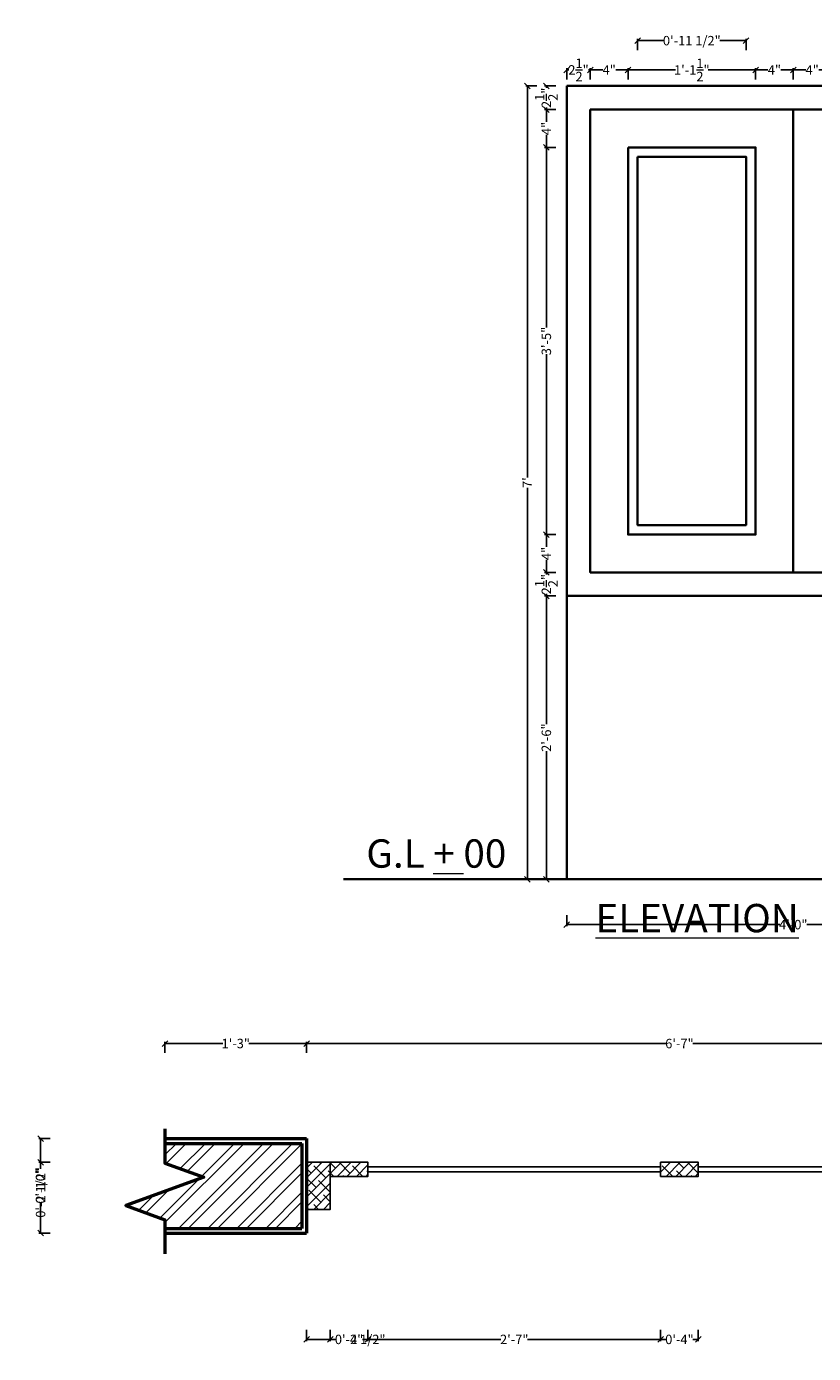
# Model space of a CAD drawing. Units: inches. Extents: x -54 to 163, y -154 to 48.
# Tile 1 of 3: x -54 to 30, y -112 to 28. Entities that reach past the tile are written whole.
import ezdxf

# ---------------------------------------------------------------- set-up
doc = ezdxf.new("R2010")
doc.units = ezdxf.units.IN
doc.header["$MEASUREMENT"] = 0
for name, color, linetype, lineweight in [('A-ANNO-DIMS', 2, 'Continuous', 18), ('A-ANNO-TEXT', 3, 'Continuous', 18), ('A-ELEV', 7, 'Continuous', 35), ('A-GLAZ', 4, 'Continuous', 25), ('A-GLAZ-PATT', 9, 'Continuous', 13), ('A-WALL', 7, 'Continuous', 50), ('A-WALL-PATT', 8, 'Continuous', 18)]:
    doc.layers.add(name, color=color, linetype=linetype, lineweight=lineweight)
doc.styles.get("Standard").update_dxf_attribs({"font": 'arial.ttf'})
doc.dimstyles.get("Standard").update_dxf_attribs({"dimtxt": 1, "dimasz": 0.6, "dimexe": 0.18, "dimexo": 0.0625, "dimgap": 0.09, "dimtad": 0, "dimdec": 1, "dimzin": 0, "dimdsep": 46, "dimlunit": 4, "dimtxsty": 'Standard', "dimblk": 'OBLIQUE', "dimcen": 0.09, "dimadec": 0, "dimazin": 0, "dimtfac": 1, "dimtdec": 1, "dimtofl": 0, "dimtmove": 0, "dimatfit": 3, "dimfxl": 1, "dimfxlon": 1, "dimtolj": 1, "dimtzin": 0, "dimarcsym": 0})

# ---------------------------------------------------------------- blocks, each defined once
blk = doc.blocks.new('_Oblique')
at = {"color": 0, "linetype": 'ByBlock', "lineweight": -2}
blk.add_line((-0.5, -0.5), (0.5, 0.5), dxfattribs=at)
blk = doc.blocks.new('*D2')
at = {"layer": 'A-ANNO-DIMS', "color": 0, "lineweight": -2, "transparency": 16777216}
for p, q in [((3.48, 22.51), (3.48, 23.69)), ((3.48, 23.51), (3.69, 23.51)), ((5.98, 23.51), (5.77, 23.51)), ((5.98, 22.51), (5.98, 23.69))]:
    blk.add_line(p, q, dxfattribs=at)
at = {"layer": 'Defpoints', "color": 0, "transparency": 16777216}
for p in [(5.98, 23.51), (3.48, 21.81), (5.98, 19.31)]:
    blk.add_point(p, dxfattribs=at)
at = {"layer": 'A-ANNO-DIMS', "color": 0, "lineweight": -2, "transparency": 16777216, "xscale": 0.6, "yscale": 0.6, "zscale": 0.6, "rotation": 180}
blk.add_blockref('_Oblique', (3.48, 23.51), dxfattribs=at)
at = {"layer": 'A-ANNO-DIMS', "color": 0, "lineweight": -2, "transparency": 16777216, "xscale": 0.6, "yscale": 0.6, "zscale": 0.6}
blk.add_blockref('_Oblique', (5.98, 23.51), dxfattribs=at)
at = {"layer": 'A-ANNO-DIMS', "color": 0, "transparency": 16777216, "insert": (4.73, 23.51), "char_height": 1, "attachment_point": 5}
blk.add_mtext('\\A1;2{\\H1x;\\S1/2;}"', dxfattribs=at)
blk = doc.blocks.new('*D3')
at = {"layer": 'A-ANNO-DIMS', "color": 0, "lineweight": -2, "transparency": 16777216}
for p, q in [((5.98, 22.51), (5.98, 23.69)), ((5.98, 23.51), (7.3, 23.51)), ((9.98, 23.51), (8.67, 23.51)), ((9.98, 22.51), (9.98, 23.69))]:
    blk.add_line(p, q, dxfattribs=at)
at = {"layer": 'Defpoints', "color": 0, "transparency": 16777216}
for p in [(9.98, 23.51), (5.98, 19.31), (9.98, 15.31)]:
    blk.add_point(p, dxfattribs=at)
at = {"layer": 'A-ANNO-DIMS', "color": 0, "lineweight": -2, "transparency": 16777216, "xscale": 0.6, "yscale": 0.6, "zscale": 0.6, "rotation": 180}
blk.add_blockref('_Oblique', (5.98, 23.51), dxfattribs=at)
at = {"layer": 'A-ANNO-DIMS', "color": 0, "lineweight": -2, "transparency": 16777216, "xscale": 0.6, "yscale": 0.6, "zscale": 0.6}
blk.add_blockref('_Oblique', (9.98, 23.51), dxfattribs=at)
at = {"layer": 'A-ANNO-DIMS', "color": 0, "transparency": 16777216, "insert": (7.98, 23.51), "char_height": 1, "attachment_point": 5}
blk.add_mtext('\\A1;4"', dxfattribs=at)
blk = doc.blocks.new('*D4')
at = {"layer": 'A-ANNO-DIMS', "color": 0, "lineweight": -2, "transparency": 16777216}
for p, q in [((9.98, 22.51), (9.98, 23.69)), ((9.98, 23.51), (14.99, 23.51)), ((23.48, 23.51), (18.47, 23.51)), ((23.48, 22.51), (23.48, 23.69))]:
    blk.add_line(p, q, dxfattribs=at)
at = {"layer": 'Defpoints', "color": 0, "transparency": 16777216}
for p in [(23.48, 23.51), (9.98, 15.31), (23.48, 15.31)]:
    blk.add_point(p, dxfattribs=at)
at = {"layer": 'A-ANNO-DIMS', "color": 0, "lineweight": -2, "transparency": 16777216, "xscale": 0.6, "yscale": 0.6, "zscale": 0.6, "rotation": 180}
blk.add_blockref('_Oblique', (9.98, 23.51), dxfattribs=at)
at = {"layer": 'A-ANNO-DIMS', "color": 0, "lineweight": -2, "transparency": 16777216, "xscale": 0.6, "yscale": 0.6, "zscale": 0.6}
blk.add_blockref('_Oblique', (23.48, 23.51), dxfattribs=at)
at = {"layer": 'A-ANNO-DIMS', "color": 0, "transparency": 16777216, "insert": (16.73, 23.51), "char_height": 1, "attachment_point": 5}
blk.add_mtext('\\A1;1\'-1{\\H1x;\\S1/2;}"', dxfattribs=at)
blk = doc.blocks.new('*D5')
at = {"layer": 'A-ANNO-DIMS', "color": 0, "lineweight": -2, "transparency": 16777216}
for p, q in [((23.48, 22.51), (23.48, 23.69)), ((23.48, 23.51), (24.8, 23.51)), ((27.48, 23.51), (26.17, 23.51)), ((27.48, 22.51), (27.48, 23.69))]:
    blk.add_line(p, q, dxfattribs=at)
at = {"layer": 'Defpoints', "color": 0, "transparency": 16777216}
for p in [(27.48, 23.51), (23.48, 15.31), (27.48, 15.31)]:
    blk.add_point(p, dxfattribs=at)
at = {"layer": 'A-ANNO-DIMS', "color": 0, "lineweight": -2, "transparency": 16777216, "xscale": 0.6, "yscale": 0.6, "zscale": 0.6, "rotation": 180}
blk.add_blockref('_Oblique', (23.48, 23.51), dxfattribs=at)
at = {"layer": 'A-ANNO-DIMS', "color": 0, "lineweight": -2, "transparency": 16777216, "xscale": 0.6, "yscale": 0.6, "zscale": 0.6}
blk.add_blockref('_Oblique', (27.48, 23.51), dxfattribs=at)
at = {"layer": 'A-ANNO-DIMS', "color": 0, "transparency": 16777216, "insert": (25.48, 23.51), "char_height": 1, "attachment_point": 5}
blk.add_mtext('\\A1;4"', dxfattribs=at)
blk = doc.blocks.new('*D6')
at = {"layer": 'A-ANNO-DIMS', "color": 0, "lineweight": -2, "transparency": 16777216}
for p, q in [((27.48, 22.51), (27.48, 23.69)), ((27.48, 23.51), (28.8, 23.51)), ((31.48, 23.51), (30.17, 23.51)), ((31.48, 22.51), (31.48, 23.69))]:
    blk.add_line(p, q, dxfattribs=at)
at = {"layer": 'Defpoints', "color": 0, "transparency": 16777216}
for p in [(31.48, 23.51), (27.48, 15.31), (31.48, 15.31)]:
    blk.add_point(p, dxfattribs=at)
at = {"layer": 'A-ANNO-DIMS', "color": 0, "lineweight": -2, "transparency": 16777216, "xscale": 0.6, "yscale": 0.6, "zscale": 0.6, "rotation": 180}
blk.add_blockref('_Oblique', (27.48, 23.51), dxfattribs=at)
at = {"layer": 'A-ANNO-DIMS', "color": 0, "lineweight": -2, "transparency": 16777216, "xscale": 0.6, "yscale": 0.6, "zscale": 0.6}
blk.add_blockref('_Oblique', (31.48, 23.51), dxfattribs=at)
at = {"layer": 'A-ANNO-DIMS', "color": 0, "transparency": 16777216, "insert": (29.48, 23.51), "char_height": 1, "attachment_point": 5}
blk.add_mtext('\\A1;4"', dxfattribs=at)
blk = doc.blocks.new('*D10')
at = {"layer": 'A-ANNO-DIMS', "color": 0, "lineweight": -2, "transparency": 16777216}
for p, q in [((2.32, 21.81), (1.14, 21.81)), ((1.32, 21.81), (1.32, 21.6)), ((2.32, 19.31), (1.14, 19.31)), ((1.32, 19.31), (1.32, 19.53))]:
    blk.add_line(p, q, dxfattribs=at)
at = {"layer": 'Defpoints', "color": 0, "transparency": 16777216}
for p in [(1.32, 21.81), (5.98, 21.81), (5.98, 19.31)]:
    blk.add_point(p, dxfattribs=at)
at = {"layer": 'A-ANNO-DIMS', "color": 0, "lineweight": -2, "transparency": 16777216, "xscale": 0.6, "yscale": 0.6, "zscale": 0.6}
for p, rotation in [((1.32, 21.81), 90), ((1.32, 19.31), 270)]:
    blk.add_blockref('_Oblique', p, dxfattribs=dict(at, rotation=rotation))
at = {"layer": 'A-ANNO-DIMS', "color": 0, "transparency": 16777216, "insert": (1.32, 20.56), "char_height": 1, "attachment_point": 5, "rotation": 90}
blk.add_mtext('\\A1;2{\\H1x;\\S1/2;}"', dxfattribs=at)
blk = doc.blocks.new('*D11')
at = {"layer": 'A-ANNO-DIMS', "color": 0, "lineweight": -2, "transparency": 16777216}
for p, q in [((2.32, 19.31), (1.14, 19.31)), ((1.32, 19.31), (1.32, 18)), ((1.32, 15.31), (1.32, 16.63)), ((2.32, 15.31), (1.14, 15.31))]:
    blk.add_line(p, q, dxfattribs=at)
at = {"layer": 'Defpoints', "color": 0, "transparency": 16777216}
for p in [(1.32, 19.31), (9.98, 19.31), (9.98, 15.31)]:
    blk.add_point(p, dxfattribs=at)
at = {"layer": 'A-ANNO-DIMS', "color": 0, "lineweight": -2, "transparency": 16777216, "xscale": 0.6, "yscale": 0.6, "zscale": 0.6}
for p, rotation in [((1.32, 19.31), 90), ((1.32, 15.31), 270)]:
    blk.add_blockref('_Oblique', p, dxfattribs=dict(at, rotation=rotation))
at = {"layer": 'A-ANNO-DIMS', "color": 0, "transparency": 16777216, "insert": (1.32, 17.31), "char_height": 1, "attachment_point": 5, "rotation": 90}
blk.add_mtext('\\A1;4"', dxfattribs=at)
blk = doc.blocks.new('*D12')
at = {"layer": 'A-ANNO-DIMS', "color": 0, "lineweight": -2, "transparency": 16777216}
for p, q in [((2.32, 15.31), (1.14, 15.31)), ((1.32, 15.31), (1.32, -3.77)), ((1.32, -25.69), (1.32, -6.6)), ((2.32, -25.69), (1.14, -25.69))]:
    blk.add_line(p, q, dxfattribs=at)
at = {"layer": 'Defpoints', "color": 0, "transparency": 16777216}
for p in [(9.98, 15.31), (1.32, -25.69), (9.98, -25.69)]:
    blk.add_point(p, dxfattribs=at)
at = {"layer": 'A-ANNO-DIMS', "color": 0, "lineweight": -2, "transparency": 16777216, "xscale": 0.6, "yscale": 0.6, "zscale": 0.6}
for p, rotation in [((1.32, 15.31), 90), ((1.32, -25.69), 270)]:
    blk.add_blockref('_Oblique', p, dxfattribs=dict(at, rotation=rotation))
at = {"layer": 'A-ANNO-DIMS', "color": 0, "transparency": 16777216, "insert": (1.32, -5.19), "char_height": 1, "attachment_point": 5, "rotation": 90}
blk.add_mtext('\\A1;3\'-5"', dxfattribs=at)
blk = doc.blocks.new('*D13')
at = {"layer": 'A-ANNO-DIMS', "color": 0, "lineweight": -2, "transparency": 16777216}
for p, q in [((2.32, -25.69), (1.14, -25.69)), ((1.32, -25.69), (1.32, -27)), ((1.32, -29.69), (1.32, -28.37)), ((2.32, -29.69), (1.14, -29.69))]:
    blk.add_line(p, q, dxfattribs=at)
at = {"layer": 'Defpoints', "color": 0, "transparency": 16777216}
for p in [(10.03, -25.69), (1.32, -29.69), (10.03, -29.69)]:
    blk.add_point(p, dxfattribs=at)
at = {"layer": 'A-ANNO-DIMS', "color": 0, "lineweight": -2, "transparency": 16777216, "xscale": 0.6, "yscale": 0.6, "zscale": 0.6}
for p, rotation in [((1.32, -25.69), 90), ((1.32, -29.69), 270)]:
    blk.add_blockref('_Oblique', p, dxfattribs=dict(at, rotation=rotation))
at = {"layer": 'A-ANNO-DIMS', "color": 0, "transparency": 16777216, "insert": (1.32, -27.69), "char_height": 1, "attachment_point": 5, "rotation": 90}
blk.add_mtext('\\A1;4"', dxfattribs=at)
blk = doc.blocks.new('*D14')
at = {"layer": 'A-ANNO-DIMS', "color": 0, "lineweight": -2, "transparency": 16777216}
for p, q in [((2.32, -29.69), (1.14, -29.69)), ((1.32, -29.69), (1.32, -29.9)), ((2.32, -32.19), (1.14, -32.19)), ((1.32, -32.19), (1.32, -31.97))]:
    blk.add_line(p, q, dxfattribs=at)
at = {"layer": 'Defpoints', "color": 0, "transparency": 16777216}
for p in [(1.32, -29.69), (5.98, -29.69), (6.04, -32.19)]:
    blk.add_point(p, dxfattribs=at)
at = {"layer": 'A-ANNO-DIMS', "color": 0, "lineweight": -2, "transparency": 16777216, "xscale": 0.6, "yscale": 0.6, "zscale": 0.6}
for p, rotation in [((1.32, -29.69), 90), ((1.32, -32.19), 270)]:
    blk.add_blockref('_Oblique', p, dxfattribs=dict(at, rotation=rotation))
at = {"layer": 'A-ANNO-DIMS', "color": 0, "transparency": 16777216, "insert": (1.32, -30.94), "char_height": 1, "attachment_point": 5, "rotation": 90}
blk.add_mtext('\\A1;2{\\H1x;\\S1/2;}"', dxfattribs=at)
blk = doc.blocks.new('*D15')
at = {"layer": 'A-ANNO-DIMS', "color": 0, "lineweight": -2, "transparency": 16777216}
for p, q in [((2.32, -32.19), (1.14, -32.19)), ((1.32, -32.19), (1.32, -45.76)), ((1.32, -62.19), (1.32, -48.61)), ((2.32, -62.19), (1.14, -62.19))]:
    blk.add_line(p, q, dxfattribs=at)
at = {"layer": 'Defpoints', "color": 0, "transparency": 16777216}
for p in [(3.48, -32.19), (1.32, -62.19), (3.48, -62.19)]:
    blk.add_point(p, dxfattribs=at)
at = {"layer": 'A-ANNO-DIMS', "color": 0, "lineweight": -2, "transparency": 16777216, "xscale": 0.6, "yscale": 0.6, "zscale": 0.6}
for p, rotation in [((1.32, -32.19), 90), ((1.32, -62.19), 270)]:
    blk.add_blockref('_Oblique', p, dxfattribs=dict(at, rotation=rotation))
at = {"layer": 'A-ANNO-DIMS', "color": 0, "transparency": 16777216, "insert": (1.32, -47.19), "char_height": 1, "attachment_point": 5, "rotation": 90}
blk.add_mtext('\\A1;2\'-6"', dxfattribs=at)
blk = doc.blocks.new('*D16')
at = {"layer": 'A-ANNO-DIMS', "color": 0, "lineweight": -2, "transparency": 16777216}
for p, q in [((0.31, 21.81), (-0.87, 21.81)), ((-0.69, 21.81), (-0.69, -19.64)), ((-0.69, -62.19), (-0.69, -20.73)), ((0.31, -62.19), (-0.87, -62.19))]:
    blk.add_line(p, q, dxfattribs=at)
at = {"layer": 'Defpoints', "color": 0, "transparency": 16777216}
for p in [(-0.69, 21.81), (3.48, 21.81), (3.48, -62.19)]:
    blk.add_point(p, dxfattribs=at)
at = {"layer": 'A-ANNO-DIMS', "color": 0, "lineweight": -2, "transparency": 16777216, "xscale": 0.6, "yscale": 0.6, "zscale": 0.6}
for p, rotation in [((-0.69, 21.81), 90), ((-0.69, -62.19), 270)]:
    blk.add_blockref('_Oblique', p, dxfattribs=dict(at, rotation=rotation))
at = {"layer": 'A-ANNO-DIMS', "color": 0, "transparency": 16777216, "insert": (-0.69, -20.19), "char_height": 1, "attachment_point": 5, "rotation": 90}
blk.add_mtext("\\A1;7'", dxfattribs=at)
blk = doc.blocks.new('*D18')
at = {"layer": 'A-ANNO-DIMS', "color": 0, "lineweight": -2, "transparency": 16777216}
for p, q in [((3.48, -65.99), (3.48, -67.17)), ((51.48, -65.99), (51.48, -67.17)), ((3.48, -66.99), (26.04, -66.99)), ((51.48, -66.99), (28.92, -66.99))]:
    blk.add_line(p, q, dxfattribs=at)
at = {"layer": 'Defpoints', "color": 0, "transparency": 16777216}
for p in [(3.48, -62.19), (51.48, -62.19), (51.48, -66.99)]:
    blk.add_point(p, dxfattribs=at)
at = {"layer": 'A-ANNO-DIMS', "color": 0, "lineweight": -2, "transparency": 16777216, "xscale": 0.6, "yscale": 0.6, "zscale": 0.6, "rotation": 180}
blk.add_blockref('_Oblique', (3.48, -66.99), dxfattribs=at)
at = {"layer": 'A-ANNO-DIMS', "color": 0, "lineweight": -2, "transparency": 16777216, "xscale": 0.6, "yscale": 0.6, "zscale": 0.6}
blk.add_blockref('_Oblique', (51.48, -66.99), dxfattribs=at)
at = {"layer": 'A-ANNO-DIMS', "color": 0, "transparency": 16777216, "insert": (27.48, -66.99), "char_height": 1, "attachment_point": 5}
blk.add_mtext('\\A1;4\'-0"', dxfattribs=at)
blk = doc.blocks.new('*D19')
at = {"layer": 'A-ANNO-DIMS', "color": 0, "lineweight": -2, "transparency": 16777216}
for p, q in [((10.98, 25.61), (10.98, 26.79)), ((22.48, 25.61), (22.48, 26.79)), ((10.98, 26.61), (13.76, 26.61)), ((22.48, 26.61), (19.7, 26.61))]:
    blk.add_line(p, q, dxfattribs=at)
at = {"layer": 'Defpoints', "color": 0, "transparency": 16777216}
for p in [(22.48, 26.61), (10.98, 14.31), (22.48, 14.31)]:
    blk.add_point(p, dxfattribs=at)
at = {"layer": 'A-ANNO-DIMS', "color": 0, "lineweight": -2, "transparency": 16777216, "xscale": 0.6, "yscale": 0.6, "zscale": 0.6, "rotation": 180}
blk.add_blockref('_Oblique', (10.98, 26.61), dxfattribs=at)
at = {"layer": 'A-ANNO-DIMS', "color": 0, "lineweight": -2, "transparency": 16777216, "xscale": 0.6, "yscale": 0.6, "zscale": 0.6}
blk.add_blockref('_Oblique', (22.48, 26.61), dxfattribs=at)
at = {"layer": 'A-ANNO-DIMS', "color": 0, "transparency": 16777216, "insert": (16.73, 26.61), "char_height": 1, "attachment_point": 5}
blk.add_mtext('\\A1;0\'-11 1/2"', dxfattribs=at)
blk = doc.blocks.new('*D20')
at = {"layer": 'A-ANNO-DIMS', "color": 0, "lineweight": -2, "transparency": 16777216}
for p, q in [((55.28, 14.31), (56.46, 14.31)), ((56.28, 14.31), (56.28, -3.77)), ((56.28, -24.69), (56.28, -6.6)), ((55.28, -24.69), (56.46, -24.69))]:
    blk.add_line(p, q, dxfattribs=at)
at = {"layer": 'Defpoints', "color": 0, "transparency": 16777216}
for p in [(10.98, 14.31), (10.98, -24.69), (56.28, -24.69)]:
    blk.add_point(p, dxfattribs=at)
at = {"layer": 'A-ANNO-DIMS', "color": 0, "lineweight": -2, "transparency": 16777216, "xscale": 0.6, "yscale": 0.6, "zscale": 0.6}
for p, rotation in [((56.28, 14.31), 90), ((56.28, -24.69), 270)]:
    blk.add_blockref('_Oblique', p, dxfattribs=dict(at, rotation=rotation))
at = {"layer": 'A-ANNO-DIMS', "color": 0, "transparency": 16777216, "insert": (56.28, -5.19), "char_height": 1, "attachment_point": 5, "rotation": 90}
blk.add_mtext('\\A1;3\'-3"', dxfattribs=at)
blk = doc.blocks.new('*D33')
at = {"layer": 'A-ANNO-DIMS', "color": 0, "lineweight": -2, "transparency": 16777216}
for p, q in [((-39.08, -80.58), (-39.08, -79.4)), ((-39.08, -79.58), (-32.96, -79.58)), ((-24.08, -79.58), (-30.21, -79.58)), ((-24.08, -80.58), (-24.08, -79.4))]:
    blk.add_line(p, q, dxfattribs=at)
at = {"layer": 'Defpoints', "color": 0, "transparency": 16777216}
for p in [(-24.08, -79.58), (-39.08, -89.65), (-24.08, -89.65)]:
    blk.add_point(p, dxfattribs=at)
at = {"layer": 'A-ANNO-DIMS', "color": 0, "lineweight": -2, "transparency": 16777216, "xscale": 0.6, "yscale": 0.6, "zscale": 0.6, "rotation": 180}
blk.add_blockref('_Oblique', (-39.08, -79.58), dxfattribs=at)
at = {"layer": 'A-ANNO-DIMS', "color": 0, "lineweight": -2, "transparency": 16777216, "xscale": 0.6, "yscale": 0.6, "zscale": 0.6}
blk.add_blockref('_Oblique', (-24.08, -79.58), dxfattribs=at)
at = {"layer": 'A-ANNO-DIMS', "color": 0, "transparency": 16777216, "insert": (-31.58, -79.58), "char_height": 1, "attachment_point": 5}
blk.add_mtext('\\A1;1\'-3"', dxfattribs=at)
blk = doc.blocks.new('*D34')
at = {"layer": 'A-ANNO-DIMS', "color": 0, "lineweight": -2, "transparency": 16777216}
for p, q in [((-24.08, -80.58), (-24.08, -79.4)), ((-24.08, -79.58), (13.99, -79.58)), ((54.92, -79.58), (16.84, -79.58)), ((54.92, -80.58), (54.92, -79.4))]:
    blk.add_line(p, q, dxfattribs=at)
at = {"layer": 'Defpoints', "color": 0, "transparency": 16777216}
for p in [(54.92, -79.58), (-24.08, -89.65), (54.92, -89.65)]:
    blk.add_point(p, dxfattribs=at)
at = {"layer": 'A-ANNO-DIMS', "color": 0, "lineweight": -2, "transparency": 16777216, "xscale": 0.6, "yscale": 0.6, "zscale": 0.6, "rotation": 180}
blk.add_blockref('_Oblique', (-24.08, -79.58), dxfattribs=at)
at = {"layer": 'A-ANNO-DIMS', "color": 0, "lineweight": -2, "transparency": 16777216, "xscale": 0.6, "yscale": 0.6, "zscale": 0.6}
blk.add_blockref('_Oblique', (54.92, -79.58), dxfattribs=at)
at = {"layer": 'A-ANNO-DIMS', "color": 0, "transparency": 16777216, "insert": (15.42, -79.58), "char_height": 1, "attachment_point": 5}
blk.add_mtext('\\A1;6\'-7"', dxfattribs=at)
blk = doc.blocks.new('*D36')
at = {"layer": 'A-ANNO-DIMS', "color": 0, "lineweight": -2, "transparency": 16777216}
for p, q in [((-24.08, -109.91), (-24.08, -111.09)), ((-24.08, -110.91), (-21.58, -110.91)), ((-21.58, -109.91), (-21.58, -111.09)), ((-21.58, -110.91), (-20.98, -110.91))]:
    blk.add_line(p, q, dxfattribs=at)
at = {"layer": 'Defpoints', "color": 0, "transparency": 16777216}
for p in [(-24.08, -97.15), (-21.58, -97.15), (-21.58, -110.91)]:
    blk.add_point(p, dxfattribs=at)
at = {"layer": 'A-ANNO-DIMS', "color": 0, "lineweight": -2, "transparency": 16777216, "xscale": 0.6, "yscale": 0.6, "zscale": 0.6, "rotation": 180}
blk.add_blockref('_Oblique', (-24.08, -110.91), dxfattribs=at)
at = {"layer": 'A-ANNO-DIMS', "color": 0, "lineweight": -2, "transparency": 16777216, "xscale": 0.6, "yscale": 0.6, "zscale": 0.6}
blk.add_blockref('_Oblique', (-21.58, -110.91), dxfattribs=at)
at = {"layer": 'A-ANNO-DIMS', "color": 0, "transparency": 16777216, "insert": (-18.4, -110.91), "char_height": 1, "attachment_point": 5}
blk.add_mtext('\\A1;0\'-2 1/2"', dxfattribs=at)
blk = doc.blocks.new('*D37')
at = {"layer": 'A-ANNO-DIMS', "color": 0, "lineweight": -2, "transparency": 16777216}
for p, q in [((-21.58, -109.91), (-21.58, -111.09)), ((-21.58, -110.91), (-21, -110.91)), ((-17.58, -110.91), (-18.17, -110.91)), ((-17.58, -109.91), (-17.58, -111.09))]:
    blk.add_line(p, q, dxfattribs=at)
at = {"layer": 'Defpoints', "color": 0, "transparency": 16777216}
for p in [(-21.58, -93.65), (-17.58, -93.65), (-17.58, -110.91)]:
    blk.add_point(p, dxfattribs=at)
at = {"layer": 'A-ANNO-DIMS', "color": 0, "lineweight": -2, "transparency": 16777216, "xscale": 0.6, "yscale": 0.6, "zscale": 0.6, "rotation": 180}
blk.add_blockref('_Oblique', (-21.58, -110.91), dxfattribs=at)
at = {"layer": 'A-ANNO-DIMS', "color": 0, "lineweight": -2, "transparency": 16777216, "xscale": 0.6, "yscale": 0.6, "zscale": 0.6}
blk.add_blockref('_Oblique', (-17.58, -110.91), dxfattribs=at)
at = {"layer": 'A-ANNO-DIMS', "color": 0, "transparency": 16777216, "insert": (-19.58, -110.91), "char_height": 1, "attachment_point": 5}
blk.add_mtext('\\A1;0\'-4"', dxfattribs=at)
blk = doc.blocks.new('*D38')
at = {"layer": 'A-ANNO-DIMS', "color": 0, "lineweight": -2, "transparency": 16777216}
for p, q in [((-17.58, -109.91), (-17.58, -111.09)), ((-17.58, -110.91), (-3.51, -110.91)), ((13.42, -110.91), (-0.66, -110.91)), ((13.42, -109.91), (13.42, -111.09))]:
    blk.add_line(p, q, dxfattribs=at)
at = {"layer": 'Defpoints', "color": 0, "transparency": 16777216}
for p in [(-17.58, -93.65), (13.42, -93.65), (13.42, -110.91)]:
    blk.add_point(p, dxfattribs=at)
at = {"layer": 'A-ANNO-DIMS', "color": 0, "lineweight": -2, "transparency": 16777216, "xscale": 0.6, "yscale": 0.6, "zscale": 0.6, "rotation": 180}
blk.add_blockref('_Oblique', (-17.58, -110.91), dxfattribs=at)
at = {"layer": 'A-ANNO-DIMS', "color": 0, "lineweight": -2, "transparency": 16777216, "xscale": 0.6, "yscale": 0.6, "zscale": 0.6}
blk.add_blockref('_Oblique', (13.42, -110.91), dxfattribs=at)
at = {"layer": 'A-ANNO-DIMS', "color": 0, "transparency": 16777216, "insert": (-2.08, -110.91), "char_height": 1, "attachment_point": 5}
blk.add_mtext('\\A1;2\'-7"', dxfattribs=at)
blk = doc.blocks.new('*D39')
at = {"layer": 'A-ANNO-DIMS', "color": 0, "lineweight": -2, "transparency": 16777216}
for p, q in [((13.42, -109.91), (13.42, -111.09)), ((13.42, -110.91), (14, -110.91)), ((17.42, -110.91), (16.83, -110.91)), ((17.42, -109.91), (17.42, -111.09))]:
    blk.add_line(p, q, dxfattribs=at)
at = {"layer": 'Defpoints', "color": 0, "transparency": 16777216}
for p in [(13.42, -93.65), (17.42, -93.65), (17.42, -110.91)]:
    blk.add_point(p, dxfattribs=at)
at = {"layer": 'A-ANNO-DIMS', "color": 0, "lineweight": -2, "transparency": 16777216, "xscale": 0.6, "yscale": 0.6, "zscale": 0.6, "rotation": 180}
blk.add_blockref('_Oblique', (13.42, -110.91), dxfattribs=at)
at = {"layer": 'A-ANNO-DIMS', "color": 0, "lineweight": -2, "transparency": 16777216, "xscale": 0.6, "yscale": 0.6, "zscale": 0.6}
blk.add_blockref('_Oblique', (17.42, -110.91), dxfattribs=at)
at = {"layer": 'A-ANNO-DIMS', "color": 0, "transparency": 16777216, "insert": (15.42, -110.91), "char_height": 1, "attachment_point": 5}
blk.add_mtext('\\A1;0\'-4"', dxfattribs=at)
blk = doc.blocks.new('*D40')
at = {"layer": 'A-ANNO-DIMS', "color": 0, "lineweight": -2, "transparency": 16777216}
for p, q in [((-51.26, -89.65), (-52.44, -89.65)), ((-52.26, -89.65), (-52.26, -92.85)), ((-52.26, -99.65), (-52.26, -96.46)), ((-51.26, -99.65), (-52.44, -99.65))]:
    blk.add_line(p, q, dxfattribs=at)
at = {"layer": 'Defpoints', "color": 0, "transparency": 16777216}
for p in [(-39.08, -89.65), (-52.26, -99.65), (-39.08, -99.65)]:
    blk.add_point(p, dxfattribs=at)
at = {"layer": 'A-ANNO-DIMS', "color": 0, "lineweight": -2, "transparency": 16777216, "xscale": 0.6, "yscale": 0.6, "zscale": 0.6}
for p, rotation in [((-52.26, -89.65), 90), ((-52.26, -99.65), 270)]:
    blk.add_blockref('_Oblique', p, dxfattribs=dict(at, rotation=rotation))
at = {"layer": 'A-ANNO-DIMS', "color": 0, "transparency": 16777216, "insert": (-52.26, -94.65), "char_height": 1, "attachment_point": 5, "rotation": 90}
blk.add_mtext('\\A1;0\'-10"', dxfattribs=at)
blk = doc.blocks.new('*D41')
at = {"layer": 'A-ANNO-DIMS', "color": 0, "lineweight": -2, "transparency": 16777216}
for p, q in [((-51.26, -89.65), (-52.44, -89.65)), ((-52.26, -89.65), (-52.26, -92.15)), ((-51.26, -92.15), (-52.44, -92.15)), ((-52.26, -92.15), (-52.26, -92.75))]:
    blk.add_line(p, q, dxfattribs=at)
at = {"layer": 'Defpoints', "color": 0, "transparency": 16777216}
for p in [(54.92, -89.65), (-52.26, -92.15), (52.42, -92.15)]:
    blk.add_point(p, dxfattribs=at)
at = {"layer": 'A-ANNO-DIMS', "color": 0, "lineweight": -2, "transparency": 16777216, "xscale": 0.6, "yscale": 0.6, "zscale": 0.6}
for p, rotation in [((-52.26, -89.65), 90), ((-52.26, -92.15), 270)]:
    blk.add_blockref('_Oblique', p, dxfattribs=dict(at, rotation=rotation))
at = {"layer": 'A-ANNO-DIMS', "color": 0, "transparency": 16777216, "insert": (-52.26, -95.34), "char_height": 1, "attachment_point": 5, "rotation": 90}
blk.add_mtext('\\A1;0\'-2 1/2"', dxfattribs=at)
blk = doc.blocks.new('*D42')
at = {"layer": 'A-ANNO-DIMS', "color": 0, "lineweight": -2, "transparency": 16777216}
for p, q in [((82.09, -92.15), (83.27, -92.15)), ((83.09, -92.15), (83.09, -93.24)), ((83.09, -97.15), (83.09, -96.07)), ((82.09, -97.15), (83.27, -97.15))]:
    blk.add_line(p, q, dxfattribs=at)
at = {"layer": 'Defpoints', "color": 0, "transparency": 16777216}
for p in [(-24.08, -92.15), (-24.08, -97.15), (83.09, -97.15)]:
    blk.add_point(p, dxfattribs=at)
at = {"layer": 'A-ANNO-DIMS', "color": 0, "lineweight": -2, "transparency": 16777216, "xscale": 0.6, "yscale": 0.6, "zscale": 0.6}
for p, rotation in [((83.09, -92.15), 90), ((83.09, -97.15), 270)]:
    blk.add_blockref('_Oblique', p, dxfattribs=dict(at, rotation=rotation))
at = {"layer": 'A-ANNO-DIMS', "color": 0, "transparency": 16777216, "insert": (83.09, -94.65), "char_height": 1, "attachment_point": 5, "rotation": 90}
blk.add_mtext('\\A1;0\'-5"', dxfattribs=at)

msp = doc.modelspace()

# ---------------------------------------------------------------- hatches: boundary and pattern name
at = {"layer": 'A-GLAZ-PATT'}
h = msp.add_hatch(dxfattribs=at)
h.set_pattern_fill('ANSI38', color=256, scale=5.8)
h.paths.add_polyline_path([(54.92, -92.15), (52.42, -92.15), (52.42, -97.15), (54.92, -97.15)])
h.paths.add_polyline_path([(52.42, -92.15), (48.42, -92.15), (48.42, -93.65), (52.42, -93.65)])
h.paths.add_polyline_path([(17.42, -92.15), (13.42, -92.15), (13.42, -93.65), (17.42, -93.65)])
h.paths.add_polyline_path([(-21.58, -92.15), (-24.08, -92.15), (-24.08, -97.15), (-21.58, -97.15)])
h.paths.add_polyline_path([(-17.58, -92.15), (-21.58, -92.15), (-21.58, -93.65), (-17.58, -93.65)])
at = {"layer": 'A-WALL-PATT'}
h = msp.add_hatch(dxfattribs=at)
h.set_pattern_fill('ANSI32', color=256, scale=5.8)
h.paths.add_polyline_path([(65.79, -93.74), (69.92, -92.24), (69.92, -90.15), (55.42, -90.15), (55.42, -99.15), (69.92, -99.15), (69.92, -98.24), (74.04, -96.74)])
h.paths.add_polyline_path([(-24.58, -90.15), (-39.08, -90.15), (-39.08, -92.24), (-34.96, -93.74), (-43.21, -96.74), (-39.08, -98.24), (-39.08, -99.15), (-24.58, -99.15)])

# ---------------------------------------------------------------- linework, layer by layer
at = {"layer": 'A-ELEV'}
for p, q in [((27.48, 19.31), (27.48, -29.69)), ((3.48, -32.19), (3.48, -62.19)), ((-20.18, -62.19), (51.48, -62.19))]:
    msp.add_line(p, q, dxfattribs=at)
msp.add_lwpolyline([(3.48, 21.81), (51.48, 21.81), (51.48, 19.31), (51.48, -29.69), (51.48, -32.19), (3.48, -32.19), (3.48, 21.81)], dxfattribs=at)
for points in [[(5.98, 19.31), (48.98, 19.31), (48.98, -29.69), (5.98, -29.69)], [(9.98, 15.31), (23.48, 15.31), (23.48, -25.69), (9.98, -25.69)], [(10.98, 14.31), (22.48, 14.31), (22.48, -24.69), (10.98, -24.69)]]:
    msp.add_lwpolyline(points, close=True, dxfattribs=at)
at = {"layer": 'A-GLAZ'}
for points in [[(-24.08, -92.15), (-24.08, -97.15), (-21.58, -97.15), (-21.58, -92.15)], [(-21.58, -92.15), (-21.58, -93.65), (-17.58, -93.65), (-17.58, -92.15)], [(-17.58, -92.65), (-17.58, -93.15), (13.42, -93.15), (13.42, -92.65)], [(13.42, -93.65), (13.42, -92.15), (17.42, -92.15), (17.42, -93.65)], [(48.42, -92.65), (48.42, -93.15), (17.42, -93.15), (17.42, -92.65)]]:
    msp.add_lwpolyline(points, close=True, dxfattribs=at)
at = {"layer": 'A-WALL'}
for p, q in [((-39.08, -89.65), (-24.08, -89.65)), ((-24.08, -89.65), (-24.08, -99.65)), ((-39.08, -90.15), (-24.58, -90.15)), ((-24.58, -90.15), (-24.58, -99.15)), ((-39.08, -99.15), (-24.58, -99.15)), ((-39.08, -99.65), (-24.08, -99.65))]:
    msp.add_line(p, q, dxfattribs=at)
msp.add_lwpolyline([(-39.08, -88.63), (-39.08, -92.24), (-34.96, -93.74), (-43.21, -96.74), (-39.08, -98.24), (-39.08, -101.86)], dxfattribs=at)

# ---------------------------------------------------------------- texts
at = {"layer": 'A-ANNO-TEXT', "char_height": 3, "attachment_point": 1}
for s, insert in [('G.L {\\L+} 00', (-17.75, -57.96)), ('{\\LELEVATION}', (6.53, -64.8))]:
    msp.add_mtext_dynamic_manual_height_columns(s, width=23.7975, gutter_width=1, heights=[0], dxfattribs=dict(at, insert=insert))

# ---------------------------------------------------------------- dimensions: what is measured, and where the dimension line sits
at = {"layer": 'A-ANNO-DIMS'}
for base, p1, p2, override, picture, middle in [((22.48, 26.61), (10.98, 14.31), (22.48, 14.31), {"dimdec": 1, "dimlfac": 1, "dimrnd": 0, "dimzin": 1, "dimdsep": 46, "dimlunit": 4, "dimfrac": 2}, '*D19', (16.73, 26.61)), ((5.98, 23.51), (3.48, 21.81), (5.98, 19.31), {"dimclrd": 0, "dimclre": 0, "dimclrt": 0}, '*D2', (4.73, 23.51)), ((9.98, 23.51), (5.98, 19.31), (9.98, 15.31), {"dimclrd": 0, "dimclre": 0, "dimclrt": 0}, '*D3', (7.98, 23.51)), ((23.48, 23.51), (9.98, 15.31), (23.48, 15.31), {"dimclrd": 0, "dimclre": 0, "dimclrt": 0}, '*D4', (16.73, 23.51)), ((27.48, 23.51), (23.48, 15.31), (27.48, 15.31), {"dimclrd": 0, "dimclre": 0, "dimclrt": 0}, '*D5', (25.48, 23.51)), ((31.48, 23.51), (27.48, 15.31), (31.48, 15.31), {"dimclrd": 0, "dimclre": 0, "dimclrt": 0}, '*D6', (29.48, 23.51)), ((51.48, -66.99), (3.48, -62.19), (51.48, -62.19), {"dimdec": 1, "dimlfac": 1, "dimrnd": 0, "dimzin": 1, "dimdsep": 46, "dimlunit": 4, "dimfrac": 2}, '*D18', (27.48, -66.99)), ((-24.08, -79.58), (-39.08, -89.65), (-24.08, -89.65), {"dimdec": 1, "dimlfac": 1, "dimrnd": 0, "dimzin": 1, "dimdsep": 46, "dimlunit": 4, "dimfrac": 2}, '*D33', (-31.58, -79.58)), ((54.92, -79.58), (-24.08, -89.65), (54.92, -89.65), {"dimdec": 1, "dimlfac": 1, "dimrnd": 0, "dimzin": 1, "dimdsep": 46, "dimlunit": 4, "dimfrac": 2}, '*D34', (15.42, -79.58)), ((-17.58, -110.91), (-21.58, -93.65), (-17.58, -93.65), {"dimdec": 1, "dimlfac": 1, "dimrnd": 0, "dimzin": 1, "dimdsep": 46, "dimlunit": 4, "dimfrac": 2}, '*D37', (-19.58, -110.91)), ((13.42, -110.91), (-17.58, -93.65), (13.42, -93.65), {"dimdec": 1, "dimlfac": 1, "dimrnd": 0, "dimzin": 1, "dimdsep": 46, "dimlunit": 4, "dimfrac": 2}, '*D38', (-2.08, -110.91)), ((17.42, -110.91), (13.42, -93.65), (17.42, -93.65), {"dimdec": 1, "dimlfac": 1, "dimrnd": 0, "dimzin": 1, "dimdsep": 46, "dimlunit": 4, "dimfrac": 2}, '*D39', (15.42, -110.91)), ((-21.58, -110.91), (-24.08, -97.15), (-21.58, -97.15), {"dimdec": 1, "dimlfac": 1, "dimrnd": 0, "dimzin": 1, "dimdsep": 46, "dimlunit": 4, "dimfrac": 2}, '*D36', (-18.4, -110.91))]:
    dim = msp.add_linear_dim(base=base, p1=p1, p2=p2, dimstyle='Standard', override=override, dxfattribs=at)
    dim.commit()
    dim.dimension.update_dxf_attribs({"geometry": picture, "text_midpoint": middle})
for base, p1, p2, override, picture, middle in [((-0.69, 21.81), (3.48, -62.19), (3.48, 21.81), {"dimclrd": 0, "dimclre": 0, "dimclrt": 0}, '*D16', (-0.69, -20.19)), ((1.32, 21.81), (5.98, 19.31), (5.98, 21.81), {"dimclrd": 0, "dimclre": 0, "dimclrt": 0}, '*D10', (1.32, 20.56)), ((1.32, 19.31), (9.98, 15.31), (9.98, 19.31), {"dimclrd": 0, "dimclre": 0, "dimclrt": 0}, '*D11', (1.32, 17.31)), ((1.32, -25.69), (9.98, 15.31), (9.98, -25.69), {"dimclrd": 0, "dimclre": 0, "dimclrt": 0}, '*D12', (1.32, -5.19)), ((56.28, -24.69), (10.98, 14.31), (10.98, -24.69), {"dimdec": 1, "dimlfac": 1, "dimrnd": 0, "dimzin": 1, "dimdsep": 46, "dimlunit": 4, "dimfrac": 2}, '*D20', (56.28, -5.19)), ((1.32, -29.69), (10.03, -25.69), (10.03, -29.69), {"dimclrd": 0, "dimclre": 0, "dimclrt": 0}, '*D13', (1.32, -27.69)), ((1.32, -29.69), (6.04, -32.19), (5.98, -29.69), {"dimclrd": 0, "dimclre": 0, "dimclrt": 0}, '*D14', (1.32, -30.94)), ((1.32, -62.19), (3.48, -32.19), (3.48, -62.19), {"dimclrd": 0, "dimclre": 0, "dimclrt": 0}, '*D15', (1.32, -47.19)), ((-52.26, -92.15), (54.92, -89.65), (52.42, -92.15), {"dimdec": 1, "dimlfac": 1, "dimrnd": 0, "dimzin": 1, "dimdsep": 46, "dimlunit": 4, "dimfrac": 2}, '*D41', (-52.26, -95.34)), ((-52.26, -99.65), (-39.08, -89.65), (-39.08, -99.65), {"dimdec": 1, "dimlfac": 1, "dimrnd": 0, "dimzin": 1, "dimdsep": 46, "dimlunit": 4, "dimfrac": 2}, '*D40', (-52.26, -94.65)), ((83.09, -97.15), (-24.08, -92.15), (-24.08, -97.15), {"dimdec": 1, "dimlfac": 1, "dimrnd": 0, "dimzin": 1, "dimdsep": 46, "dimlunit": 4, "dimfrac": 2}, '*D42', (83.09, -94.65))]:
    dim = msp.add_linear_dim(base=base, p1=p1, p2=p2, angle=90, dimstyle='Standard', override=override, dxfattribs=at)
    dim.commit()
    dim.dimension.update_dxf_attribs({"geometry": picture, "text_midpoint": middle})

doc.saveas('drawing.dxf')
